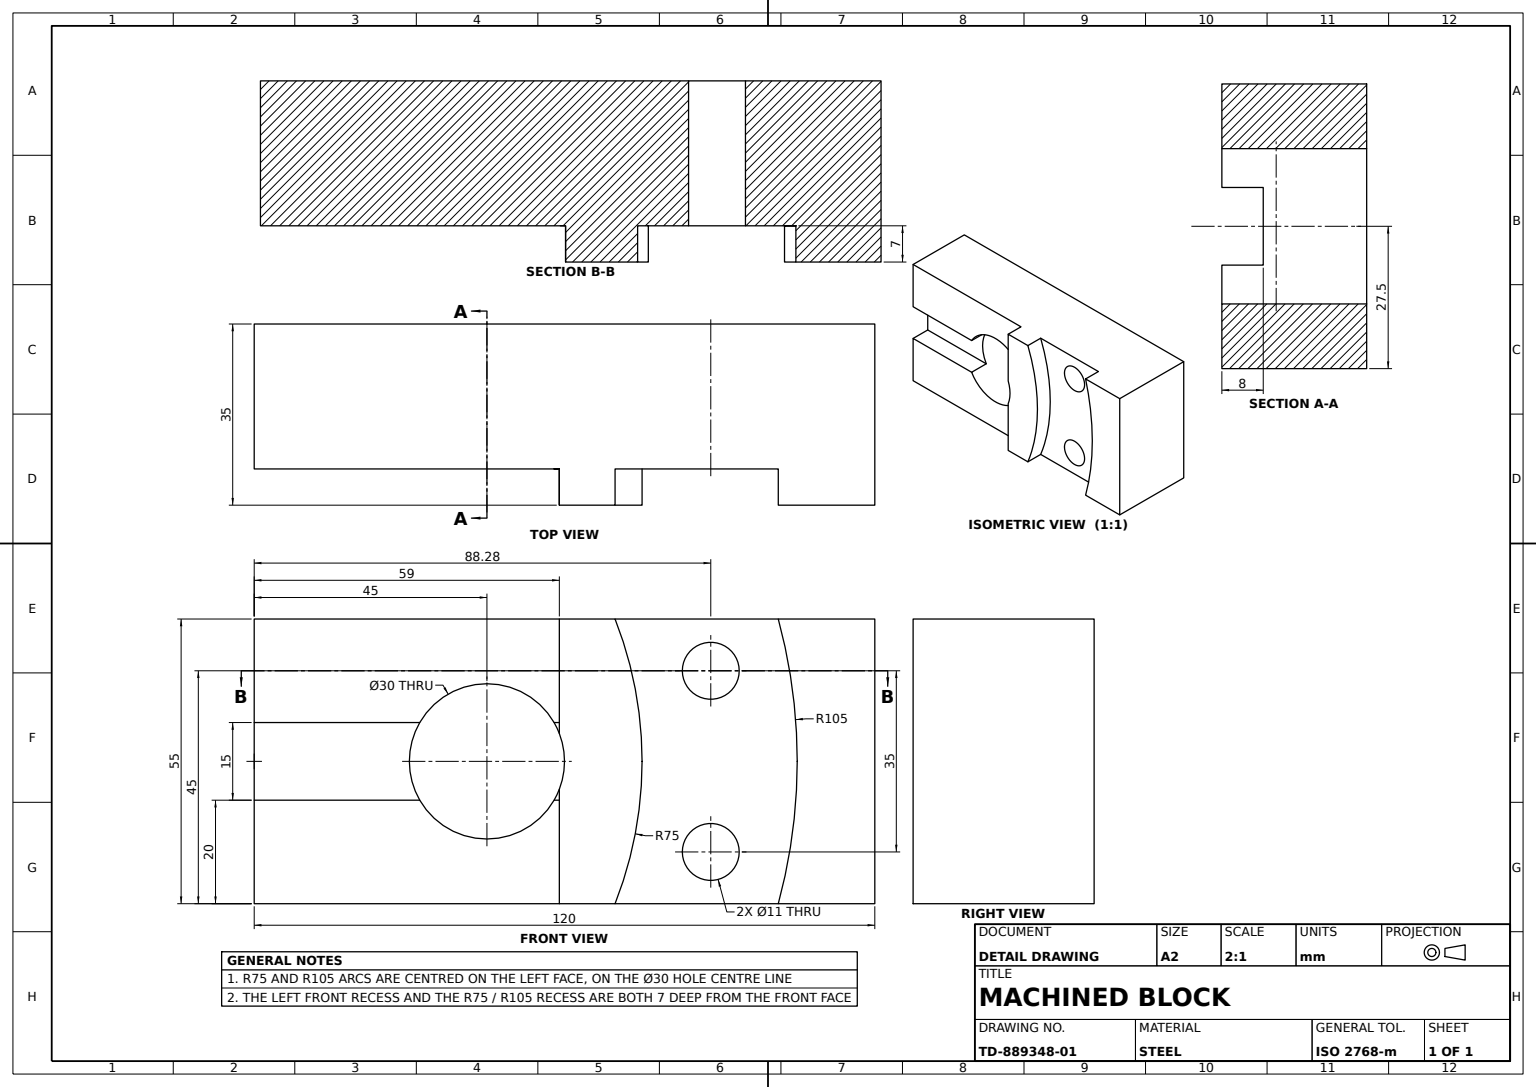
SolidWorks part; units mm, degrees
material "Plain Carbon Steel"
ref_plane "Front Plane" through (0, 0, 0) normal (0, 0, 1) x (1, 0, 0)
ref_plane "Top Plane" through (0, 0, 0) normal (0, 1, 0) x (1, 0, 0)
ref_plane "Right Plane" through (0, 0, 0) normal (1, 0, 0) x (0, 0, -1)
sketch "Slide Profile Sketch" plane through (0, 0, 0) normal (0, 0, 1) x (1, 0, 0)
  line L0 (-60, 27.5) -> (89.8581, 27.5) construction
  line L1 (-60, 0) -> (60, 0)
  line L2 (-60, 0) -> (-60, 55)
  line L3 (-60, 55) -> (60, 55)
  line L4 (60, 0) -> (60, 55)
  circle A0 centre (-15, 27.5) radius 15
  circle A1 centre (-60, 27.5) radius 90 construction
  circle A2 centre (28.2822, 45) radius 5.5
  circle A3 centre (28.2822, 10) radius 5.5
  point P4 (0, 0)
  dimension "D3" = 30
  dimension "D5" = 180
  dimension "D7" = 11
  dimension "D1" = 120
  dimension "D2" = 55
  dimension "D4" = 45
  dimension "D6" = 35
extrude "Slide Body 35mm" add sketch "Slide Profile Sketch" along normal blind 35
sketch "Face Recess Sketch" plane through (0, 0, 35) normal (0, 0, 1) x (1, 0, 0)
  line L0 (-60, 55) -> (-60, 0) construction
  line L1 (9.7764, 55) -> (41.3348, 55)
  line L2 (60, 55) -> (-60, 55) construction
  line L3 (9.7764, 0) -> (41.3348, 0)
  line L4 (-60, 0) -> (60, 0) construction
  arc A0 (9.7764, 0) -> (9.7764, 55) centre (-60, 27.5) ccw
  arc A1 (41.3348, 0) -> (41.3348, 55) centre (-60, 27.5) ccw
  dimension "D1" = 150
  dimension "D2" = 210
extrude "Face Recess 7mm" cut sketch "Face Recess Sketch" against normal blind 7
sketch "Curved Pocket Sketch" plane through (0, 0, 35) normal (0, 0, 1) x (1, 0, 0)
  line L0 (9.7764, 55) -> (-60, 55) construction
  line L1 (-60, 0) -> (-1, 0)
  line L2 (-60, 0) -> (-60, 55)
  line L3 (-60, 55) -> (-1, 55)
  line L4 (-1, 0) -> (-1, 55)
  dimension "D1" = 59
extrude "Curved Pocket 7mm" cut sketch "Curved Pocket Sketch" against normal blind 7
sketch "Through Cut Sketch" plane through (-60, 0, 0) normal (-1, 0, 0) x (0, 0, 1)
  line L0 (0, 27.5) -> (46.4931, 27.5) construction
  line L1 (0, 55) -> (0, 0) construction
  line L2 (28, 0) -> (28, 22.1148) construction
  line L3 (28, 20) -> (20, 20)
  line L4 (28, 20) -> (28, 35)
  line L5 (28, 35) -> (20, 35)
  line L6 (20, 20) -> (20, 35)
  point P10 (28, 27.5)
  dimension "D1" = 20
  dimension "D2" = 15
extrude "Through Cut 59mm" cut sketch "Through Cut Sketch" against normal blind 59
